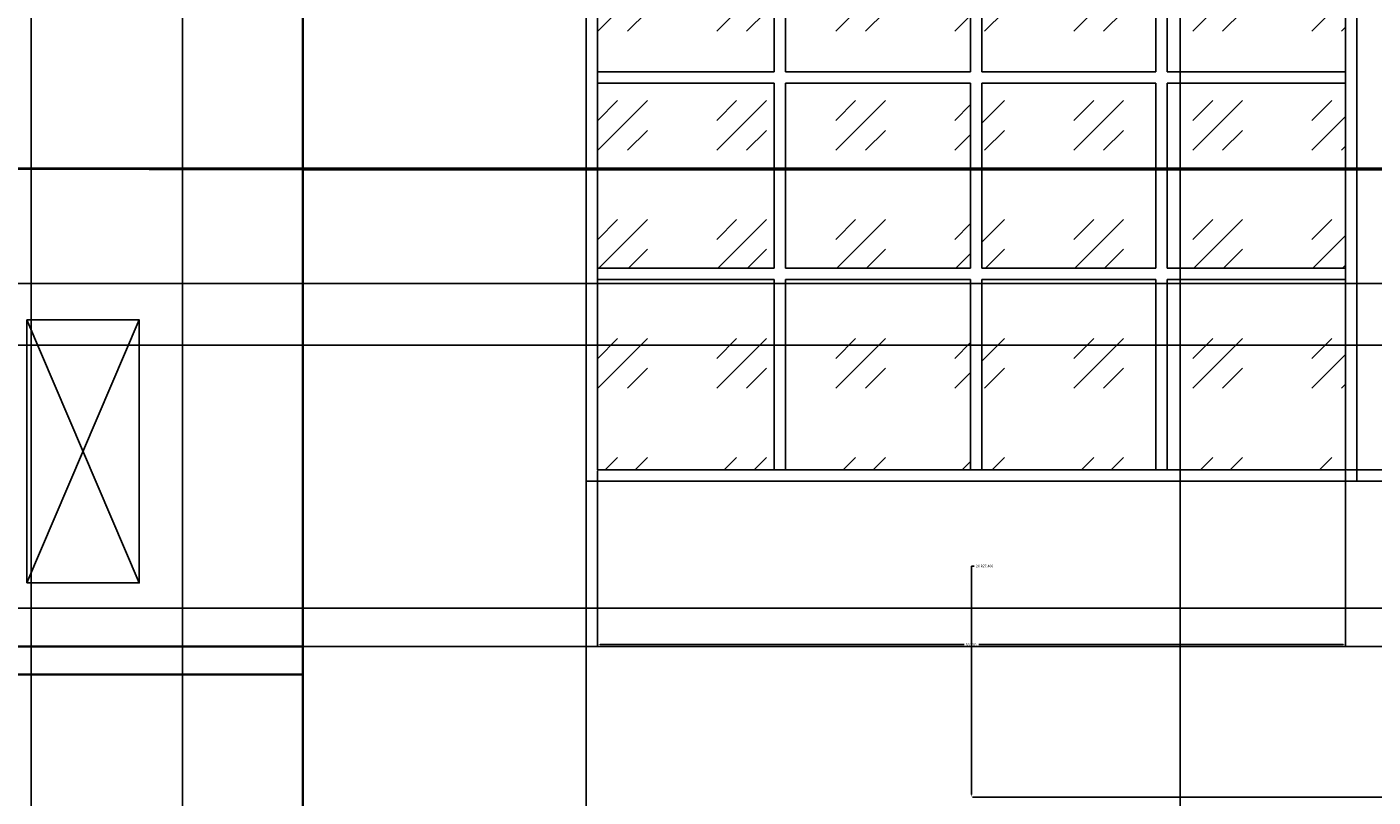
# Model space of a CAD drawing. Units: inches. Extents: x 93 to 565, y 123 to 656.
# Tile 14 of 18: x 418 to 513, y 463 to 518. Entities that reach past the tile are written whole.
import ezdxf

# ---------------------------------------------------------------- set-up
doc = ezdxf.new("R2010")
doc.units = ezdxf.units.IN
doc.header["$MEASUREMENT"] = 0
for name, color, linetype, lineweight in [('A-ANNO-DIMS', 2, 'Continuous', 18), ('A-ELEV', 7, 'Continuous', 35), ('A-GLAZ', 4, 'Continuous', 25)]:
    doc.layers.add(name, color=color, linetype=linetype, lineweight=lineweight)
doc.styles.get("Standard").update_dxf_attribs({"font": 'arial.ttf'})
doc.dimstyles.get("Standard").update_dxf_attribs({"dimtxt": 0.18, "dimasz": 0.18, "dimexe": 0.18, "dimexo": 0.0625, "dimgap": 0.09, "dimtad": 0, "dimtih": 1, "dimtoh": 1, "dimdec": 4, "dimzin": 0, "dimdsep": 46, "dimtxsty": 'Standard', "dimcen": 0.09, "dimadec": 0, "dimazin": 0, "dimtfac": 1, "dimtdec": 4, "dimtofl": 0, "dimtmove": 0, "dimatfit": 3, "dimfxl": 1, "dimtolj": 1, "dimtzin": 0, "dimarcsym": 0})

# ---------------------------------------------------------------- blocks, each defined once
blk = doc.blocks.new('*U9')
for p, q in [((0, 0), (38, 89)), ((38, 0), (0, 89))]:
    blk.add_line(p, q)
blk.add_lwpolyline([(0, 0), (38, 0), (38, 89), (0, 89)], close=True)
blk = doc.blocks.new('WIN-ARCHED')
for p, q in [((26.666, 83.051), (26.666, 70.384)), ((27.466, 83.039), (27.466, 70.358)), ((3.385, 69.387), (14.576, 63.554)), ((3.006, 68.683), (14.186, 62.855)), ((50.181, 68.96), (38.77, 63.306)), ((50.548, 68.249), (39.145, 62.599)), ((0, 56.384), (12.6, 56.384)), ((0, 56.384), (0.2, 56.384)), ((0, 56.384), (0, 32.384)), ((13.4, 56.384), (39.8, 56.384)), ((40.6, 56.384), (53.333, 56.384)), ((0, 55.584), (12.6, 55.584)), ((12.6, 55.584), (12.6, 42.384)), ((13.4, 55.584), (13.4, 42.384)), ((13.4, 55.584), (26.6, 55.584)), ((26.6, 55.584), (26.6, 42.384)), ((27.4, 55.584), (27.4, 42.384)), ((27.4, 55.584), (39.8, 55.584)), ((39.8, 55.584), (39.8, 42.384)), ((40.6, 55.584), (40.6, 42.384)), ((40.6, 55.584), (53.333, 55.584)), ((0, 42.384), (12.6, 42.384)), ((13.4, 42.384), (26.6, 42.384)), ((27.4, 42.384), (39.8, 42.384)), ((40.6, 42.384), (53.333, 42.384)), ((0, 41.584), (12.6, 41.584)), ((12.6, 41.584), (12.6, 28.384)), ((13.4, 41.584), (13.4, 28.384)), ((13.4, 41.584), (26.6, 41.584)), ((26.6, 41.584), (26.6, 28.384)), ((27.4, 41.584), (27.4, 28.384)), ((27.4, 41.584), (39.8, 41.584)), ((39.8, 41.584), (39.8, 28.384)), ((40.6, 41.584), (40.6, 28.384)), ((40.6, 41.584), (53.333, 41.584)), ((0, 28.384), (12.6, 28.384)), ((13.4, 28.384), (26.6, 28.384)), ((27.4, 28.384), (39.8, 28.384)), ((40.6, 28.384), (53.333, 28.384)), ((0, 27.584), (12.6, 27.584)), ((12.6, 27.584), (12.6, 14.384)), ((13.4, 27.584), (13.4, 14.384)), ((13.4, 27.584), (26.6, 27.584)), ((26.6, 27.584), (26.6, 14.384)), ((27.4, 27.584), (27.4, 14.384)), ((27.4, 27.584), (39.8, 27.584)), ((39.8, 27.584), (39.8, 14.384)), ((40.6, 27.584), (40.6, 14.384)), ((40.6, 27.584), (53.333, 27.584)), ((0, 14.384), (12.6, 14.384)), ((0, 13.584), (12.6, 13.584)), ((12.6, 13.584), (12.6, 0)), ((13.4, 14.384), (26.6, 14.384)), ((13.4, 13.584), (13.4, 0)), ((13.4, 13.584), (26.6, 13.584)), ((26.6, 13.584), (26.6, 0)), ((27.4, 14.384), (39.8, 14.384)), ((27.4, 13.584), (27.4, 0)), ((27.4, 13.584), (39.8, 13.584)), ((39.8, 13.584), (39.8, 0)), ((40.6, 14.384), (53.333, 14.384)), ((40.6, 13.584), (40.6, 0)), ((40.6, 13.584), (53.333, 13.584))]:
    blk.add_line(p, q)
blk.add_lwpolyline([(53.333, 56.384), (53.333, 0), (0, 0), (0, 56.384)])
for centre, radius, start, end in [((26.666, 56.384), 26.666, 90, 150.81666), ((26.666, 56.384), 26.666, 28.13721, 88.28084), ((26.6, 56.384), 14, 89.72913, 149.19423), ((26.6, 56.384), 14, 29.63071, 86.45282), ((26.6, 56.384), 13.2, 0, 180), ((26.666, 56.384), 26.666, 152.53579, 180), ((26.666, 56.384), 26.666, 0, 26.41802), ((26.6, 56.384), 14, 152.47006, 180), ((26.6, 56.384), 14, 0, 26.35489)]:
    blk.add_arc(centre, radius, start, end)
blk = doc.blocks.new('*D20')
at = {"layer": 'A-ANNO-DIMS', "color": 0, "lineweight": -2, "transparency": 16777216}
for p, q in [((511.588, 569.373), (524.163, 569.373)), ((523.983, 569.193), (523.983, 528.031)), ((523.983, 486.502), (523.983, 527.664)), ((511.588, 486.322), (524.163, 486.322))]:
    blk.add_line(p, q, dxfattribs=at)
at = {"layer": 'A-ANNO-DIMS', "color": 0, "transparency": 16777216}
for points in [[(523.953, 569.193), (524.013, 569.193), (523.983, 569.373)], [(523.953, 486.502), (524.013, 486.502), (523.983, 486.322)]]:
    blk.add_solid(points, dxfattribs=at)
at = {"layer": 'Defpoints', "color": 0, "transparency": 16777216}
for p in [(511.526, 569.373), (523.983, 569.373), (511.526, 486.322)]:
    blk.add_point(p, dxfattribs=at)
at = {"layer": 'A-ANNO-DIMS', "color": 0, "transparency": 16777216, "insert": (523.983, 527.847), "char_height": 0.18, "attachment_point": 5}
blk.add_mtext('\\A1;ARCHED WINDOW 83 TYP.', dxfattribs=at)
blk = doc.blocks.new('*D21')
at = {"layer": 'A-ANNO-DIMS', "color": 0, "lineweight": -2, "transparency": 16777216}
for p, q in [((458.193, 486.26), (458.193, 473.685)), ((511.526, 486.26), (511.526, 473.685)), ((458.373, 473.865), (484.331, 473.865)), ((511.346, 473.865), (485.388, 473.865))]:
    blk.add_line(p, q, dxfattribs=at)
at = {"layer": 'A-ANNO-DIMS', "color": 0, "transparency": 16777216}
for points in [[(458.373, 473.895), (458.373, 473.835), (458.193, 473.865)], [(511.346, 473.895), (511.346, 473.835), (511.526, 473.865)]]:
    blk.add_solid(points, dxfattribs=at)
at = {"layer": 'Defpoints', "color": 0, "transparency": 16777216}
for p in [(458.193, 486.322), (511.526, 486.322), (511.526, 473.865)]:
    blk.add_point(p, dxfattribs=at)
at = {"layer": 'A-ANNO-DIMS', "color": 0, "transparency": 16777216, "insert": (484.859, 473.865), "char_height": 0.18, "attachment_point": 5}
blk.add_mtext('\\A1;53 TYP.', dxfattribs=at)
blk = doc.blocks.new('*D29')
at = {"layer": 'A-ANNO-DIMS', "color": 0, "lineweight": -2, "transparency": 16777216}
for p, q in [((437.189, 594.342), (437.189, 134.002)), ((295.687, 183.67), (295.687, 134.002)), ((295.867, 134.182), (366.052, 134.182)), ((437.009, 134.182), (366.824, 134.182))]:
    blk.add_line(p, q, dxfattribs=at)
at = {"layer": 'A-ANNO-DIMS', "color": 0, "transparency": 16777216}
for points in [[(295.867, 134.212), (295.867, 134.152), (295.687, 134.182)], [(437.009, 134.212), (437.009, 134.152), (437.189, 134.182)]]:
    blk.add_solid(points, dxfattribs=at)
at = {"layer": 'Defpoints', "color": 0, "transparency": 16777216}
for p in [(437.189, 594.405), (295.687, 183.732), (437.189, 134.182)]:
    blk.add_point(p, dxfattribs=at)
at = {"layer": 'A-ANNO-DIMS', "color": 0, "transparency": 16777216, "insert": (366.438, 134.182), "char_height": 0.18, "attachment_point": 5}
blk.add_mtext('\\A1;141.5', dxfattribs=at)
blk = doc.blocks.new('*D30')
at = {"layer": 'A-ANNO-DIMS', "color": 0, "lineweight": -2, "transparency": 16777216}
for p, q in [((437.189, 594.342), (437.189, 134.002)), ((539.079, 159.67), (539.079, 134.002)), ((437.369, 134.182), (487.749, 134.182)), ((538.899, 134.182), (488.519, 134.182))]:
    blk.add_line(p, q, dxfattribs=at)
at = {"layer": 'A-ANNO-DIMS', "color": 0, "transparency": 16777216}
for points in [[(437.369, 134.212), (437.369, 134.152), (437.189, 134.182)], [(538.899, 134.212), (538.899, 134.152), (539.079, 134.182)]]:
    blk.add_solid(points, dxfattribs=at)
at = {"layer": 'Defpoints', "color": 0, "transparency": 16777216}
for p in [(437.189, 594.405), (539.079, 159.732), (539.079, 134.182)]:
    blk.add_point(p, dxfattribs=at)
at = {"layer": 'A-ANNO-DIMS', "color": 0, "transparency": 16777216, "insert": (488.134, 134.182), "char_height": 0.18, "attachment_point": 5}
blk.add_mtext('\\A1;101.9', dxfattribs=at)
blk = doc.blocks.new('*D31')
at = {"layer": 'A-ANNO-DIMS', "color": 0, "lineweight": -2, "transparency": 16777216}
for p, q in [((417.872, 630.405), (564.809, 630.405)), ((564.629, 630.225), (564.629, 395.25)), ((564.629, 159.912), (564.629, 394.887)), ((119.142, 159.732), (564.809, 159.732))]:
    blk.add_line(p, q, dxfattribs=at)
at = {"layer": 'A-ANNO-DIMS', "color": 0, "transparency": 16777216}
for points in [[(564.599, 630.225), (564.659, 630.225), (564.629, 630.405)], [(564.599, 159.912), (564.659, 159.912), (564.629, 159.732)]]:
    blk.add_solid(points, dxfattribs=at)
at = {"layer": 'Defpoints', "color": 0, "transparency": 16777216}
for p in [(417.81, 630.405), (564.629, 630.405), (119.079, 159.732)]:
    blk.add_point(p, dxfattribs=at)
at = {"layer": 'A-ANNO-DIMS', "color": 0, "transparency": 16777216, "insert": (564.629, 395.069), "char_height": 0.18, "attachment_point": 5}
blk.add_mtext('\\A1;470.7', dxfattribs=at)
blk = doc.blocks.new('*D69')
at = {"layer": 'A-ANNO-DIMS', "color": 0, "lineweight": -2, "transparency": 16777216}
for p, q in [((355.46, 420.63), (355.46, 656.135)), ((355.64, 655.955), (391.645, 655.955)), ((428.436, 655.955), (392.431, 655.955)), ((428.616, 420.63), (428.616, 656.135))]:
    blk.add_line(p, q, dxfattribs=at)
at = {"layer": 'A-ANNO-DIMS', "color": 0, "transparency": 16777216}
for points in [[(355.64, 655.985), (355.64, 655.925), (355.46, 655.955)], [(428.436, 655.985), (428.436, 655.925), (428.616, 655.955)]]:
    blk.add_solid(points, dxfattribs=at)
at = {"layer": 'Defpoints', "color": 0, "transparency": 16777216}
for p in [(428.616, 655.955), (355.46, 420.567), (428.616, 420.567)]:
    blk.add_point(p, dxfattribs=at)
at = {"layer": 'A-ANNO-DIMS', "color": 0, "transparency": 16777216, "insert": (392.038, 655.955), "char_height": 0.18, "attachment_point": 5}
blk.add_mtext('\\A1;73.16', dxfattribs=at)
blk = doc.blocks.new('*D73')
at = {"layer": 'A-ANNO-DIMS', "color": 0, "lineweight": -2, "transparency": 16777216}
for p, q in [((437.251, 473.732), (564.809, 473.732)), ((564.629, 473.552), (564.629, 460.914)), ((564.629, 447.912), (564.629, 460.55)), ((437.251, 447.732), (564.809, 447.732))]:
    blk.add_line(p, q, dxfattribs=at)
at = {"layer": 'A-ANNO-DIMS', "color": 0, "transparency": 16777216}
for points in [[(564.599, 473.552), (564.659, 473.552), (564.629, 473.732)], [(564.599, 447.912), (564.659, 447.912), (564.629, 447.732)]]:
    blk.add_solid(points, dxfattribs=at)
at = {"layer": 'Defpoints', "color": 0, "transparency": 16777216}
for p in [(437.189, 473.732), (564.629, 473.732), (437.189, 447.732)]:
    blk.add_point(p, dxfattribs=at)
at = {"layer": 'A-ANNO-DIMS', "color": 0, "transparency": 16777216, "insert": (564.629, 460.732), "char_height": 0.18, "attachment_point": 5}
blk.add_mtext('\\A1;26', dxfattribs=at)
blk = doc.blocks.new('*D74')
at = {"layer": 'A-ANNO-DIMS', "color": 0, "lineweight": -2, "transparency": 16777216}
for p, q in [((437.251, 507.732), (564.809, 507.732)), ((564.629, 507.552), (564.629, 490.914)), ((564.629, 473.912), (564.629, 490.55)), ((437.251, 473.732), (564.809, 473.732))]:
    blk.add_line(p, q, dxfattribs=at)
at = {"layer": 'A-ANNO-DIMS', "color": 0, "transparency": 16777216}
for points in [[(564.599, 507.552), (564.659, 507.552), (564.629, 507.732)], [(564.599, 473.912), (564.659, 473.912), (564.629, 473.732)]]:
    blk.add_solid(points, dxfattribs=at)
at = {"layer": 'Defpoints', "color": 0, "transparency": 16777216}
for p in [(437.189, 507.732), (564.629, 507.732), (437.189, 473.732)]:
    blk.add_point(p, dxfattribs=at)
at = {"layer": 'A-ANNO-DIMS', "color": 0, "transparency": 16777216, "insert": (564.629, 490.732), "char_height": 0.18, "attachment_point": 5}
blk.add_mtext('\\A1;34', dxfattribs=at)
blk = doc.blocks.new('*D76')
at = {"layer": 'A-ANNO-DIMS', "color": 0, "lineweight": -2, "transparency": 16777216}
for p, q in [((399.695, 507.892), (399.695, 656.135)), ((399.875, 655.955), (417.978, 655.955)), ((437.009, 655.955), (418.905, 655.955)), ((437.189, 507.795), (437.189, 656.135))]:
    blk.add_line(p, q, dxfattribs=at)
at = {"layer": 'A-ANNO-DIMS', "color": 0, "transparency": 16777216}
for points in [[(399.875, 655.985), (399.875, 655.925), (399.695, 655.955)], [(437.009, 655.985), (437.009, 655.925), (437.189, 655.955)]]:
    blk.add_solid(points, dxfattribs=at)
at = {"layer": 'Defpoints', "color": 0, "transparency": 16777216}
for p in [(437.189, 655.955), (399.695, 507.83), (437.189, 507.732)]:
    blk.add_point(p, dxfattribs=at)
at = {"layer": 'A-ANNO-DIMS', "color": 0, "transparency": 16777216, "insert": (418.442, 655.955), "char_height": 0.18, "attachment_point": 5}
blk.add_mtext('\\A1;37.494', dxfattribs=at)
blk = doc.blocks.new('*D77')
at = {"layer": 'A-ANNO-DIMS', "color": 0, "lineweight": -2, "transparency": 16777216}
for p, q in [((399.757, 507.83), (564.809, 507.83)), ((564.629, 507.65), (564.629, 503.901)), ((564.629, 499.789), (564.629, 503.538)), ((375.075, 499.609), (564.809, 499.609))]:
    blk.add_line(p, q, dxfattribs=at)
at = {"layer": 'A-ANNO-DIMS', "color": 0, "transparency": 16777216}
for points in [[(564.599, 507.65), (564.659, 507.65), (564.629, 507.83)], [(564.599, 499.789), (564.659, 499.789), (564.629, 499.609)]]:
    blk.add_solid(points, dxfattribs=at)
at = {"layer": 'Defpoints', "color": 0, "transparency": 16777216}
for p in [(399.695, 507.83), (564.629, 507.83), (375.012, 499.609)]:
    blk.add_point(p, dxfattribs=at)
at = {"layer": 'A-ANNO-DIMS', "color": 0, "transparency": 16777216, "insert": (564.629, 503.719), "char_height": 0.18, "attachment_point": 5}
blk.add_mtext('\\A1;8.221', dxfattribs=at)
blk = doc.blocks.new('*D79')
at = {"layer": 'A-ANNO-DIMS', "color": 0, "lineweight": -2, "transparency": 16777216}
for p, q in [((391.284, 495.217), (564.809, 495.217)), ((564.629, 495.037), (564.629, 486.022)), ((564.629, 476.644), (564.629, 485.658)), ((391.284, 476.464), (564.809, 476.464))]:
    blk.add_line(p, q, dxfattribs=at)
at = {"layer": 'A-ANNO-DIMS', "color": 0, "transparency": 16777216}
for points in [[(564.599, 495.037), (564.659, 495.037), (564.629, 495.217)], [(564.599, 476.644), (564.659, 476.644), (564.629, 476.464)]]:
    blk.add_solid(points, dxfattribs=at)
at = {"layer": 'Defpoints', "color": 0, "transparency": 16777216}
for p in [(391.222, 495.217), (564.629, 495.217), (391.222, 476.464)]:
    blk.add_point(p, dxfattribs=at)
at = {"layer": 'A-ANNO-DIMS', "color": 0, "transparency": 16777216, "insert": (564.629, 485.84), "char_height": 0.18, "attachment_point": 5}
blk.add_mtext('\\A1;18.753', dxfattribs=at)
blk = doc.blocks.new('*D82')
at = {"layer": 'A-ANNO-DIMS', "color": 0, "lineweight": -2, "transparency": 16777216}
for p, q in [((437.189, 447.795), (437.189, 656.135)), ((437.369, 655.955), (446.825, 655.955)), ((457.213, 655.955), (447.757, 655.955)), ((457.393, 378.4), (457.393, 656.135))]:
    blk.add_line(p, q, dxfattribs=at)
at = {"layer": 'A-ANNO-DIMS', "color": 0, "transparency": 16777216}
for points in [[(437.369, 655.985), (437.369, 655.925), (437.189, 655.955)], [(457.213, 655.985), (457.213, 655.925), (457.393, 655.955)]]:
    blk.add_solid(points, dxfattribs=at)
at = {"layer": 'Defpoints', "color": 0, "transparency": 16777216}
for p in [(457.393, 655.955), (437.189, 447.732), (457.393, 378.337)]:
    blk.add_point(p, dxfattribs=at)
at = {"layer": 'A-ANNO-DIMS', "color": 0, "transparency": 16777216, "insert": (447.291, 655.955), "char_height": 0.18, "attachment_point": 5}
blk.add_mtext('\\A1;20.205', dxfattribs=at)
blk = doc.blocks.new('*D85')
at = {"layer": 'A-ANNO-DIMS', "color": 0, "lineweight": -2, "transparency": 16777216}
for p, q in [((457.456, 485.522), (564.809, 485.522)), ((564.629, 485.342), (564.629, 474.437)), ((564.629, 463.168), (564.629, 474.073)), ((484.922, 462.988), (564.809, 462.988))]:
    blk.add_line(p, q, dxfattribs=at)
at = {"layer": 'A-ANNO-DIMS', "color": 0, "transparency": 16777216}
for points in [[(564.599, 485.342), (564.659, 485.342), (564.629, 485.522)], [(564.599, 463.168), (564.659, 463.168), (564.629, 462.988)]]:
    blk.add_solid(points, dxfattribs=at)
at = {"layer": 'Defpoints', "color": 0, "transparency": 16777216}
for p in [(457.393, 485.522), (564.629, 485.522), (484.859, 462.988)]:
    blk.add_point(p, dxfattribs=at)
at = {"layer": 'A-ANNO-DIMS', "color": 0, "transparency": 16777216, "insert": (564.629, 474.255), "char_height": 0.18, "attachment_point": 5}
blk.add_mtext('\\A1;22.535', dxfattribs=at)
blk = doc.blocks.new('*D90')
at = {"layer": 'A-ANNO-DIMS', "color": 0, "lineweight": -2, "transparency": 16777216}
for p, q in [((417.81, 594.342), (417.81, 134.002)), ((437.189, 594.342), (437.189, 134.002)), ((417.99, 134.182), (427.114, 134.182)), ((437.009, 134.182), (427.885, 134.182))]:
    blk.add_line(p, q, dxfattribs=at)
at = {"layer": 'A-ANNO-DIMS', "color": 0, "transparency": 16777216}
for points in [[(417.99, 134.212), (417.99, 134.152), (417.81, 134.182)], [(437.009, 134.212), (437.009, 134.152), (437.189, 134.182)]]:
    blk.add_solid(points, dxfattribs=at)
at = {"layer": 'Defpoints', "color": 0, "transparency": 16777216}
for p in [(417.81, 594.405), (437.189, 594.405), (437.189, 134.182)]:
    blk.add_point(p, dxfattribs=at)
at = {"layer": 'A-ANNO-DIMS', "color": 0, "transparency": 16777216, "insert": (427.499, 134.182), "char_height": 0.18, "attachment_point": 5}
blk.add_mtext('\\A1;19.38', dxfattribs=at)
blk = doc.blocks.new('*D91')
at = {"layer": 'A-ANNO-DIMS', "color": 0, "lineweight": -2, "transparency": 16777216}
for p, q in [((499.729, 599.755), (499.729, 134.002)), ((437.189, 594.342), (437.189, 134.002)), ((437.369, 134.182), (468.065, 134.182)), ((499.549, 134.182), (468.853, 134.182))]:
    blk.add_line(p, q, dxfattribs=at)
at = {"layer": 'A-ANNO-DIMS', "color": 0, "transparency": 16777216}
for points in [[(437.369, 134.212), (437.369, 134.152), (437.189, 134.182)], [(499.549, 134.212), (499.549, 134.152), (499.729, 134.182)]]:
    blk.add_solid(points, dxfattribs=at)
at = {"layer": 'Defpoints', "color": 0, "transparency": 16777216}
for p in [(499.729, 599.817), (437.189, 594.405), (499.729, 134.182)]:
    blk.add_point(p, dxfattribs=at)
at = {"layer": 'A-ANNO-DIMS', "color": 0, "transparency": 16777216, "insert": (468.459, 134.182), "char_height": 0.18, "attachment_point": 5}
blk.add_mtext('\\A1;62.54', dxfattribs=at)
blk = doc.blocks.new('*D92')
at = {"layer": 'A-ANNO-DIMS', "color": 0, "lineweight": -2, "transparency": 16777216}
for p, q in [((523.142, 603.135), (523.142, 134.002)), ((499.729, 599.755), (499.729, 134.002)), ((499.909, 134.182), (510.971, 134.182)), ((522.962, 134.182), (511.9, 134.182))]:
    blk.add_line(p, q, dxfattribs=at)
at = {"layer": 'A-ANNO-DIMS', "color": 0, "transparency": 16777216}
for points in [[(499.909, 134.212), (499.909, 134.152), (499.729, 134.182)], [(522.962, 134.212), (522.962, 134.152), (523.142, 134.182)]]:
    blk.add_solid(points, dxfattribs=at)
at = {"layer": 'Defpoints', "color": 0, "transparency": 16777216}
for p in [(523.142, 603.198), (499.729, 599.817), (523.142, 134.182)]:
    blk.add_point(p, dxfattribs=at)
at = {"layer": 'A-ANNO-DIMS', "color": 0, "transparency": 16777216, "insert": (511.435, 134.182), "char_height": 0.18, "attachment_point": 5}
blk.add_mtext('\\A1;23.412', dxfattribs=at)
blk = doc.blocks.new('*D101')
at = {"layer": 'A-ANNO-DIMS', "color": 0, "lineweight": -2, "transparency": 16777216}
for p, q in [((485.04, 479.467), (484.86, 479.467)), ((484.86, 479.467), (484.86, 463.168)), ((484.769, 435.521), (484.949, 435.521)), ((484.859, 435.431), (484.859, 435.611))]:
    blk.add_line(p, q, dxfattribs=at)
at = {"layer": 'A-ANNO-DIMS', "color": 0, "transparency": 16777216}
blk.add_solid([(484.83, 463.168), (484.89, 463.168), (484.86, 462.988)], dxfattribs=at)
at = {"layer": 'Defpoints', "color": 0, "transparency": 16777216}
for p in [(484.86, 462.988), (484.859, 435.521)]:
    blk.add_point(p, dxfattribs=at)
at = {"layer": 'A-ANNO-DIMS', "color": 0, "transparency": 16777216, "insert": (485.785, 479.467), "char_height": 0.18, "attachment_point": 5}
blk.add_mtext('\\A1;2X R27.466', dxfattribs=at)
blk = doc.blocks.new('*D108')
at = {"layer": 'A-ANNO-DIMS', "color": 0, "lineweight": -2, "transparency": 16777216}
for p, q in [((437.189, 594.342), (437.189, 134.002)), ((295.687, 183.67), (295.687, 134.002)), ((295.867, 134.182), (365.93, 134.182)), ((437.009, 134.182), (366.946, 134.182))]:
    blk.add_line(p, q, dxfattribs=at)
at = {"layer": 'A-ANNO-DIMS', "color": 0, "transparency": 16777216}
for points in [[(295.867, 134.212), (295.867, 134.152), (295.687, 134.182)], [(437.009, 134.212), (437.009, 134.152), (437.189, 134.182)]]:
    blk.add_solid(points, dxfattribs=at)
at = {"layer": 'Defpoints', "color": 0, "transparency": 16777216}
for p in [(437.189, 594.405), (295.687, 183.732), (437.189, 134.182)]:
    blk.add_point(p, dxfattribs=at)
at = {"layer": 'A-ANNO-DIMS', "color": 0, "transparency": 16777216, "insert": (366.438, 134.182), "char_height": 0.18, "attachment_point": 5}
blk.add_mtext('\\A1;141.501', dxfattribs=at)
blk = doc.blocks.new('*D109')
at = {"layer": 'A-ANNO-DIMS', "color": 0, "lineweight": -2, "transparency": 16777216}
for p, q in [((437.189, 594.342), (437.189, 134.002)), ((539.079, 159.67), (539.079, 134.002)), ((437.369, 134.182), (487.626, 134.182)), ((538.899, 134.182), (488.642, 134.182))]:
    blk.add_line(p, q, dxfattribs=at)
at = {"layer": 'A-ANNO-DIMS', "color": 0, "transparency": 16777216}
for points in [[(437.369, 134.212), (437.369, 134.152), (437.189, 134.182)], [(538.899, 134.212), (538.899, 134.152), (539.079, 134.182)]]:
    blk.add_solid(points, dxfattribs=at)
at = {"layer": 'Defpoints', "color": 0, "transparency": 16777216}
for p in [(437.189, 594.405), (539.079, 159.732), (539.079, 134.182)]:
    blk.add_point(p, dxfattribs=at)
at = {"layer": 'A-ANNO-DIMS', "color": 0, "transparency": 16777216, "insert": (488.134, 134.182), "char_height": 0.18, "attachment_point": 5}
blk.add_mtext('\\A1;101.891', dxfattribs=at)
blk = doc.blocks.new('*D110')
at = {"layer": 'A-ANNO-DIMS', "color": 0, "lineweight": -2, "transparency": 16777216}
for p, q in [((417.872, 630.405), (564.809, 630.405)), ((564.629, 630.225), (564.629, 395.25)), ((564.629, 159.912), (564.629, 394.887)), ((119.142, 159.732), (564.809, 159.732))]:
    blk.add_line(p, q, dxfattribs=at)
at = {"layer": 'A-ANNO-DIMS', "color": 0, "transparency": 16777216}
for points in [[(564.599, 630.225), (564.659, 630.225), (564.629, 630.405)], [(564.599, 159.912), (564.659, 159.912), (564.629, 159.732)]]:
    blk.add_solid(points, dxfattribs=at)
at = {"layer": 'Defpoints', "color": 0, "transparency": 16777216}
for p in [(417.81, 630.405), (564.629, 630.405), (119.079, 159.732)]:
    blk.add_point(p, dxfattribs=at)
at = {"layer": 'A-ANNO-DIMS', "color": 0, "transparency": 16777216, "insert": (564.629, 395.069), "char_height": 0.18, "attachment_point": 5}
blk.add_mtext('\\A1;470.673', dxfattribs=at)
blk = doc.blocks.new('*D148')
at = {"layer": 'A-ANNO-DIMS', "color": 0, "lineweight": -2, "transparency": 16777216}
for p, q in [((355.46, 420.63), (355.46, 656.135)), ((355.64, 655.955), (391.575, 655.955)), ((428.436, 655.955), (392.501, 655.955)), ((428.616, 420.63), (428.616, 656.135))]:
    blk.add_line(p, q, dxfattribs=at)
at = {"layer": 'A-ANNO-DIMS', "color": 0, "transparency": 16777216}
for points in [[(355.64, 655.985), (355.64, 655.925), (355.46, 655.955)], [(428.436, 655.985), (428.436, 655.925), (428.616, 655.955)]]:
    blk.add_solid(points, dxfattribs=at)
at = {"layer": 'Defpoints', "color": 0, "transparency": 16777216}
for p in [(428.616, 655.955), (355.46, 420.567), (428.616, 420.567)]:
    blk.add_point(p, dxfattribs=at)
at = {"layer": 'A-ANNO-DIMS', "color": 0, "transparency": 16777216, "insert": (392.038, 655.955), "char_height": 0.18, "attachment_point": 5}
blk.add_mtext('\\A1;73.156', dxfattribs=at)
blk = doc.blocks.new('*D152')
at = {"layer": 'A-ANNO-DIMS', "color": 0, "lineweight": -2, "transparency": 16777216}
for p, q in [((437.251, 473.732), (564.809, 473.732)), ((564.629, 473.552), (564.629, 460.914)), ((564.629, 447.912), (564.629, 460.55)), ((437.251, 447.732), (564.809, 447.732))]:
    blk.add_line(p, q, dxfattribs=at)
at = {"layer": 'A-ANNO-DIMS', "color": 0, "transparency": 16777216}
for points in [[(564.599, 473.552), (564.659, 473.552), (564.629, 473.732)], [(564.599, 447.912), (564.659, 447.912), (564.629, 447.732)]]:
    blk.add_solid(points, dxfattribs=at)
at = {"layer": 'Defpoints', "color": 0, "transparency": 16777216}
for p in [(437.189, 473.732), (564.629, 473.732), (437.189, 447.732)]:
    blk.add_point(p, dxfattribs=at)
at = {"layer": 'A-ANNO-DIMS', "color": 0, "transparency": 16777216, "insert": (564.629, 460.732), "char_height": 0.18, "attachment_point": 5}
blk.add_mtext('\\A1;26.000', dxfattribs=at)
blk = doc.blocks.new('*D153')
at = {"layer": 'A-ANNO-DIMS', "color": 0, "lineweight": -2, "transparency": 16777216}
for p, q in [((437.251, 507.732), (564.809, 507.732)), ((564.629, 507.552), (564.629, 490.914)), ((564.629, 473.912), (564.629, 490.55)), ((437.251, 473.732), (564.809, 473.732))]:
    blk.add_line(p, q, dxfattribs=at)
at = {"layer": 'A-ANNO-DIMS', "color": 0, "transparency": 16777216}
for points in [[(564.599, 507.552), (564.659, 507.552), (564.629, 507.732)], [(564.599, 473.912), (564.659, 473.912), (564.629, 473.732)]]:
    blk.add_solid(points, dxfattribs=at)
at = {"layer": 'Defpoints', "color": 0, "transparency": 16777216}
for p in [(437.189, 507.732), (564.629, 507.732), (437.189, 473.732)]:
    blk.add_point(p, dxfattribs=at)
at = {"layer": 'A-ANNO-DIMS', "color": 0, "transparency": 16777216, "insert": (564.629, 490.732), "char_height": 0.18, "attachment_point": 5}
blk.add_mtext('\\A1;34.000', dxfattribs=at)
blk = doc.blocks.new('*D155')
at = {"layer": 'A-ANNO-DIMS', "color": 0, "lineweight": -2, "transparency": 16777216}
for p, q in [((399.695, 507.892), (399.695, 656.135)), ((399.875, 655.955), (417.978, 655.955)), ((437.009, 655.955), (418.905, 655.955)), ((437.189, 507.795), (437.189, 656.135))]:
    blk.add_line(p, q, dxfattribs=at)
at = {"layer": 'A-ANNO-DIMS', "color": 0, "transparency": 16777216}
for points in [[(399.875, 655.985), (399.875, 655.925), (399.695, 655.955)], [(437.009, 655.985), (437.009, 655.925), (437.189, 655.955)]]:
    blk.add_solid(points, dxfattribs=at)
at = {"layer": 'Defpoints', "color": 0, "transparency": 16777216}
for p in [(437.189, 655.955), (399.695, 507.83), (437.189, 507.732)]:
    blk.add_point(p, dxfattribs=at)
at = {"layer": 'A-ANNO-DIMS', "color": 0, "transparency": 16777216, "insert": (418.442, 655.955), "char_height": 0.18, "attachment_point": 5}
blk.add_mtext('\\A1;37.494', dxfattribs=at)
blk = doc.blocks.new('*D156')
at = {"layer": 'A-ANNO-DIMS', "color": 0, "lineweight": -2, "transparency": 16777216}
for p, q in [((399.757, 507.83), (564.809, 507.83)), ((564.629, 507.65), (564.629, 503.901)), ((564.629, 499.789), (564.629, 503.538)), ((375.075, 499.609), (564.809, 499.609))]:
    blk.add_line(p, q, dxfattribs=at)
at = {"layer": 'A-ANNO-DIMS', "color": 0, "transparency": 16777216}
for points in [[(564.599, 507.65), (564.659, 507.65), (564.629, 507.83)], [(564.599, 499.789), (564.659, 499.789), (564.629, 499.609)]]:
    blk.add_solid(points, dxfattribs=at)
at = {"layer": 'Defpoints', "color": 0, "transparency": 16777216}
for p in [(399.695, 507.83), (564.629, 507.83), (375.012, 499.609)]:
    blk.add_point(p, dxfattribs=at)
at = {"layer": 'A-ANNO-DIMS', "color": 0, "transparency": 16777216, "insert": (564.629, 503.719), "char_height": 0.18, "attachment_point": 5}
blk.add_mtext('\\A1;8.221', dxfattribs=at)
blk = doc.blocks.new('*D158')
at = {"layer": 'A-ANNO-DIMS', "color": 0, "lineweight": -2, "transparency": 16777216}
for p, q in [((391.284, 495.217), (564.809, 495.217)), ((564.629, 495.037), (564.629, 486.022)), ((564.629, 476.644), (564.629, 485.658)), ((391.284, 476.464), (564.809, 476.464))]:
    blk.add_line(p, q, dxfattribs=at)
at = {"layer": 'A-ANNO-DIMS', "color": 0, "transparency": 16777216}
for points in [[(564.599, 495.037), (564.659, 495.037), (564.629, 495.217)], [(564.599, 476.644), (564.659, 476.644), (564.629, 476.464)]]:
    blk.add_solid(points, dxfattribs=at)
at = {"layer": 'Defpoints', "color": 0, "transparency": 16777216}
for p in [(391.222, 495.217), (564.629, 495.217), (391.222, 476.464)]:
    blk.add_point(p, dxfattribs=at)
at = {"layer": 'A-ANNO-DIMS', "color": 0, "transparency": 16777216, "insert": (564.629, 485.84), "char_height": 0.18, "attachment_point": 5}
blk.add_mtext('\\A1;18.753', dxfattribs=at)
blk = doc.blocks.new('*D161')
at = {"layer": 'A-ANNO-DIMS', "color": 0, "lineweight": -2, "transparency": 16777216}
for p, q in [((437.189, 447.795), (437.189, 656.135)), ((437.369, 655.955), (446.825, 655.955)), ((457.213, 655.955), (447.757, 655.955)), ((457.393, 378.4), (457.393, 656.135))]:
    blk.add_line(p, q, dxfattribs=at)
at = {"layer": 'A-ANNO-DIMS', "color": 0, "transparency": 16777216}
for points in [[(437.369, 655.985), (437.369, 655.925), (437.189, 655.955)], [(457.213, 655.985), (457.213, 655.925), (457.393, 655.955)]]:
    blk.add_solid(points, dxfattribs=at)
at = {"layer": 'Defpoints', "color": 0, "transparency": 16777216}
for p in [(457.393, 655.955), (437.189, 447.732), (457.393, 378.337)]:
    blk.add_point(p, dxfattribs=at)
at = {"layer": 'A-ANNO-DIMS', "color": 0, "transparency": 16777216, "insert": (447.291, 655.955), "char_height": 0.18, "attachment_point": 5}
blk.add_mtext('\\A1;20.205', dxfattribs=at)
blk = doc.blocks.new('*D164')
at = {"layer": 'A-ANNO-DIMS', "color": 0, "lineweight": -2, "transparency": 16777216}
for p, q in [((457.456, 485.522), (564.809, 485.522)), ((564.629, 485.342), (564.629, 474.437)), ((564.629, 463.168), (564.629, 474.073)), ((484.922, 462.988), (564.809, 462.988))]:
    blk.add_line(p, q, dxfattribs=at)
at = {"layer": 'A-ANNO-DIMS', "color": 0, "transparency": 16777216}
for points in [[(564.599, 485.342), (564.659, 485.342), (564.629, 485.522)], [(564.599, 463.168), (564.659, 463.168), (564.629, 462.988)]]:
    blk.add_solid(points, dxfattribs=at)
at = {"layer": 'Defpoints', "color": 0, "transparency": 16777216}
for p in [(457.393, 485.522), (564.629, 485.522), (484.859, 462.988)]:
    blk.add_point(p, dxfattribs=at)
at = {"layer": 'A-ANNO-DIMS', "color": 0, "transparency": 16777216, "insert": (564.629, 474.255), "char_height": 0.18, "attachment_point": 5}
blk.add_mtext('\\A1;22.535', dxfattribs=at)
blk = doc.blocks.new('*D169')
at = {"layer": 'A-ANNO-DIMS', "color": 0, "lineweight": -2, "transparency": 16777216}
for p, q in [((417.81, 594.342), (417.81, 134.002)), ((437.189, 594.342), (437.189, 134.002)), ((417.99, 134.182), (427.044, 134.182)), ((437.009, 134.182), (427.954, 134.182))]:
    blk.add_line(p, q, dxfattribs=at)
at = {"layer": 'A-ANNO-DIMS', "color": 0, "transparency": 16777216}
for points in [[(417.99, 134.212), (417.99, 134.152), (417.81, 134.182)], [(437.009, 134.212), (437.009, 134.152), (437.189, 134.182)]]:
    blk.add_solid(points, dxfattribs=at)
at = {"layer": 'Defpoints', "color": 0, "transparency": 16777216}
for p in [(417.81, 594.405), (437.189, 594.405), (437.189, 134.182)]:
    blk.add_point(p, dxfattribs=at)
at = {"layer": 'A-ANNO-DIMS', "color": 0, "transparency": 16777216, "insert": (427.499, 134.182), "char_height": 0.18, "attachment_point": 5}
blk.add_mtext('\\A1;19.379', dxfattribs=at)
blk = doc.blocks.new('*D170')
at = {"layer": 'A-ANNO-DIMS', "color": 0, "lineweight": -2, "transparency": 16777216}
for p, q in [((499.729, 599.755), (499.729, 134.002)), ((437.189, 594.342), (437.189, 134.002)), ((437.369, 134.182), (468.012, 134.182)), ((499.549, 134.182), (468.906, 134.182))]:
    blk.add_line(p, q, dxfattribs=at)
at = {"layer": 'A-ANNO-DIMS', "color": 0, "transparency": 16777216}
for points in [[(437.369, 134.212), (437.369, 134.152), (437.189, 134.182)], [(499.549, 134.212), (499.549, 134.152), (499.729, 134.182)]]:
    blk.add_solid(points, dxfattribs=at)
at = {"layer": 'Defpoints', "color": 0, "transparency": 16777216}
for p in [(499.729, 599.817), (437.189, 594.405), (499.729, 134.182)]:
    blk.add_point(p, dxfattribs=at)
at = {"layer": 'A-ANNO-DIMS', "color": 0, "transparency": 16777216, "insert": (468.459, 134.182), "char_height": 0.18, "attachment_point": 5}
blk.add_mtext('\\A1;62.541', dxfattribs=at)
blk = doc.blocks.new('*D171')
at = {"layer": 'A-ANNO-DIMS', "color": 0, "lineweight": -2, "transparency": 16777216}
for p, q in [((523.142, 603.135), (523.142, 134.002)), ((499.729, 599.755), (499.729, 134.002)), ((499.909, 134.182), (510.971, 134.182)), ((522.962, 134.182), (511.9, 134.182))]:
    blk.add_line(p, q, dxfattribs=at)
at = {"layer": 'A-ANNO-DIMS', "color": 0, "transparency": 16777216}
for points in [[(499.909, 134.212), (499.909, 134.152), (499.729, 134.182)], [(522.962, 134.212), (522.962, 134.152), (523.142, 134.182)]]:
    blk.add_solid(points, dxfattribs=at)
at = {"layer": 'Defpoints', "color": 0, "transparency": 16777216}
for p in [(523.142, 603.198), (499.729, 599.817), (523.142, 134.182)]:
    blk.add_point(p, dxfattribs=at)
at = {"layer": 'A-ANNO-DIMS', "color": 0, "transparency": 16777216, "insert": (511.435, 134.182), "char_height": 0.18, "attachment_point": 5}
blk.add_mtext('\\A1;23.412', dxfattribs=at)
blk = doc.blocks.new('*D199')
at = {"layer": 'A-ANNO-DIMS', "color": 0, "lineweight": -2, "transparency": 16777216}
for p, q in [((485.04, 479.467), (484.86, 479.467)), ((484.86, 479.467), (484.86, 463.168)), ((484.769, 435.521), (484.949, 435.521)), ((484.859, 435.431), (484.859, 435.611))]:
    blk.add_line(p, q, dxfattribs=at)
at = {"layer": 'A-ANNO-DIMS', "color": 0, "transparency": 16777216}
blk.add_solid([(484.83, 463.168), (484.89, 463.168), (484.86, 462.988)], dxfattribs=at)
at = {"layer": 'Defpoints', "color": 0, "transparency": 16777216}
for p in [(484.86, 462.988), (484.859, 435.521)]:
    blk.add_point(p, dxfattribs=at)
at = {"layer": 'A-ANNO-DIMS', "color": 0, "transparency": 16777216, "insert": (485.785, 479.467), "char_height": 0.18, "attachment_point": 5}
blk.add_mtext('\\A1;2X R27.466', dxfattribs=at)

msp = doc.modelspace()

# ---------------------------------------------------------------- hatches: boundary and pattern name
at = {"layer": 'A-GLAZ'}
h = msp.add_hatch(dxfattribs=at)
h.set_pattern_fill('GOST_GLASS', color=256)
h.set_pattern_definition([(45, (0, 0), (8.48528, 0), [5, -7]), (45, (2.1213, 0), (8.48528, 0), [2, -10]), (45, (0, 2.1213), (8.48528, 0), [2, -10])])
h.paths.add_polyline_path([(472.3785, 549.1774), (461.1986, 555.0047, 0.1204122), (458.1933, 542.7064), (458.3933, 542.7064), (470.7933, 542.7064, -0.1207031)])
h.paths.add_polyline_path([(470.7933, 541.9064), (458.1933, 541.9064), (458.1933, 528.7064), (470.7933, 528.7064)])
h.paths.add_polyline_path([(470.7933, 527.9064), (458.1933, 527.9064), (458.1933, 518.7064), (458.1933, 514.7064), (470.7933, 514.7064)])
h.paths.add_polyline_path([(470.7933, 513.9064), (458.1933, 513.9064), (458.1933, 500.7064), (470.7933, 500.7064)])
h.paths.add_polyline_path([(470.7933, 499.9064), (458.1933, 499.9064), (458.1933, 486.3222), (470.7933, 486.3222)])
h.paths.add_polyline_path([(484.7933, 499.9064), (471.5933, 499.9064), (471.5933, 486.3222), (484.7933, 486.3222)])
h.paths.add_polyline_path([(484.7933, 513.9064), (471.5933, 513.9064), (471.5933, 500.7064), (484.7933, 500.7064)])
h.paths.add_polyline_path([(484.7933, 527.9064), (471.5933, 527.9064), (471.5933, 514.7064), (484.7933, 514.7064)])
h.paths.add_polyline_path([(484.7933, 541.9064), (471.5933, 541.9064), (471.5933, 528.7064), (484.7933, 528.7064)])
h.paths.add_polyline_path([(497.9933, 541.9064), (485.5933, 541.9064), (485.5933, 528.7064), (497.9933, 528.7064)])
h.paths.add_polyline_path([(497.9933, 527.9064), (485.5933, 527.9064), (485.5933, 514.7064), (497.9933, 514.7064)])
h.paths.add_polyline_path([(497.9933, 513.9064), (485.5933, 513.9064), (485.5933, 500.7064), (497.9933, 500.7064)])
h.paths.add_polyline_path([(497.9933, 499.9064), (485.5933, 499.9064), (485.5933, 486.3222), (497.9933, 486.3222)])
h.paths.add_polyline_path([(511.5257, 499.9064), (498.7933, 499.9064), (498.7933, 486.3222), (511.5257, 486.3222)])
h.paths.add_polyline_path([(511.5257, 513.9064), (498.7933, 513.9064), (498.7933, 500.7064), (511.5257, 500.7064)])
h.paths.add_polyline_path([(511.5257, 527.9064), (498.7933, 527.9064), (498.7933, 514.7064), (511.5257, 514.7064)])
h.paths.add_polyline_path([(511.5257, 541.9064), (498.7933, 541.9064), (498.7933, 528.7064), (511.5257, 528.7064)])
h.paths.add_polyline_path([(471.5933, 542.7064), (497.9933, 542.7064, 1)])
h.paths.add_polyline_path([(508.741, 554.5706), (497.3382, 548.9214, -0.1155045), (498.7933, 542.7064), (511.5257, 542.7064, 0.1157836)])
h.paths.add_polyline_path([(485.6595, 569.3606), (485.6595, 556.6796, -0.2531415), (496.9625, 549.6281), (508.3743, 555.2818, 0.268621)])
h.paths.add_polyline_path([(484.8595, 569.3726, 0.271772), (461.5782, 555.709), (472.7686, 549.8762, -0.2654493), (484.8595, 556.7062)])

# ---------------------------------------------------------------- linework, layer by layer
at = {"layer": 'A-ELEV'}
for p, q in [((437.1885, 594.4048), (437.1885, 507.7323)), ((399.6946, 507.8299), (437.1885, 507.7323)), ((437.1885, 507.7323), (437.1885, 447.7323)), ((210.5443, 473.7323), (437.1885, 473.7323)), ((210.5443, 471.7323), (437.1885, 471.7323))]:
    msp.add_line(p, q, dxfattribs=at)
at = {"layer": 'A-GLAZ'}
msp.add_lwpolyline([(512.3257, 542.7064), (512.3257, 485.5222), (457.3933, 485.5222), (457.3933, 542.7064)], dxfattribs=at)

# ---------------------------------------------------------------- block references
msp.add_blockref('WIN-ARCHED', (458.193, 486.322), dxfattribs=at)
at = {"layer": 'A-GLAZ', "xscale": 0.2107133031769033, "yscale": 0.2107133031769033, "zscale": 0.2107133031769033}
msp.add_blockref('*U9', (417.5132, 478.2628), dxfattribs=at)

# ---------------------------------------------------------------- dimensions: what is measured, and where the dimension line sits
at = {"layer": 'A-ANNO-DIMS'}
for base, p1, p2, override, picture, middle in [((428.6158, 655.9548), (355.4603, 420.5674), (428.6158, 420.5674), {"dimdec": 2, "dimlfac": 1, "dimrnd": 0, "dimzin": 0, "dimdsep": 46, "dimlunit": 2}, '*D69', (392.038, 655.9548)), ((428.615792, 655.954775), (355.460288, 420.567351), (428.615792, 420.567351), {"dimdec": 3, "dimlfac": 1, "dimrnd": 0, "dimzin": 0, "dimdsep": 46, "dimlunit": 2}, '*D148', (392.03804, 655.954775)), ((437.1885, 655.9548), (399.6946, 507.8299), (437.1885, 507.7323), {"dimdec": 3, "dimlfac": 1, "dimrnd": 0, "dimzin": 0, "dimdsep": 46, "dimlunit": 2}, '*D76', (418.4415, 655.9548)), ((437.1885, 655.9548), (399.6946, 507.8299), (437.1885, 507.7323), {"dimdec": 3, "dimlfac": 1, "dimrnd": 0, "dimzin": 0, "dimdsep": 46, "dimlunit": 2}, '*D155', (418.4415, 655.9548)), ((457.3933, 655.9548), (437.1885, 447.7323), (457.3933, 378.3372), {"dimdec": 3, "dimlfac": 1, "dimrnd": 0, "dimzin": 0, "dimdsep": 46, "dimlunit": 2}, '*D82', (447.2909, 655.9548)), ((457.3933, 655.9548), (437.1885, 447.7323), (457.3933, 378.3372), {"dimdec": 3, "dimlfac": 1, "dimrnd": 0, "dimzin": 0, "dimdsep": 46, "dimlunit": 2}, '*D161', (447.2909, 655.9548)), ((523.1415, 134.1823), (499.7291, 599.8171), (523.1415, 603.1979), {"dimdec": 3, "dimlfac": 1, "dimrnd": 0, "dimzin": 0, "dimdsep": 46, "dimlunit": 2}, '*D92', (511.4353, 134.1823)), ((523.1415, 134.1823), (499.7291, 599.8171), (523.1415, 603.1979), {"dimdec": 3, "dimlfac": 1, "dimrnd": 0, "dimzin": 0, "dimdsep": 46, "dimlunit": 2}, '*D171', (511.4353, 134.1823)), ((499.7291, 134.1823), (437.1885, 594.4048), (499.7291, 599.8171), {"dimdec": 2, "dimlfac": 1, "dimrnd": 0, "dimzin": 0, "dimdsep": 46, "dimlunit": 2}, '*D91', (468.4588, 134.1823)), ((499.7291, 134.1823), (437.1885, 594.4048), (499.7291, 599.8171), {"dimdec": 3, "dimlfac": 1, "dimrnd": 0, "dimzin": 0, "dimdsep": 46, "dimlunit": 2}, '*D170', (468.4588, 134.1823)), ((437.1885, 134.1823), (295.6874, 183.7323), (437.1885, 594.4048), {"dimdec": 1, "dimlfac": 1, "dimrnd": 0, "dimzin": 0, "dimdsep": 46, "dimlunit": 2}, '*D29', (366.438, 134.1823)), ((437.1885, 134.1823), (295.6874, 183.7323), (437.1885, 594.4048), {"dimdec": 3, "dimlfac": 1, "dimrnd": 0, "dimzin": 0, "dimdsep": 46, "dimlunit": 2}, '*D108', (366.438, 134.1823)), ((437.1885, 134.1823), (417.8097, 594.4048), (437.1885, 594.4048), {"dimdec": 2, "dimlfac": 1, "dimrnd": 0, "dimzin": 0, "dimdsep": 46, "dimlunit": 2}, '*D90', (427.4991, 134.1823)), ((437.1885, 134.1823), (417.8097, 594.4048), (437.1885, 594.4048), {"dimdec": 3, "dimlfac": 1, "dimrnd": 0, "dimzin": 0, "dimdsep": 46, "dimlunit": 2}, '*D169', (427.4991, 134.1823)), ((539.0794, 134.1823), (437.1885, 594.4048), (539.0794, 159.7323), {"dimdec": 1, "dimlfac": 1, "dimrnd": 0, "dimzin": 0, "dimdsep": 46, "dimlunit": 2}, '*D30', (488.1339, 134.1823)), ((539.0794, 134.1823), (437.1885, 594.4048), (539.0794, 159.7323), {"dimdec": 3, "dimlfac": 1, "dimrnd": 0, "dimzin": 0, "dimdsep": 46, "dimlunit": 2}, '*D109', (488.1339, 134.1823))]:
    dim = msp.add_linear_dim(base=base, p1=p1, p2=p2, dimstyle='Standard', override=override, dxfattribs=at)
    dim.commit()
    dim.dimension.update_dxf_attribs({"geometry": picture, "text_midpoint": middle})
for base, p1, p2, override, picture, middle in [((564.6294, 630.4048), (119.0794, 159.7323), (417.8097, 630.4048), {"dimdec": 1, "dimlfac": 1, "dimrnd": 0, "dimzin": 0, "dimdsep": 46, "dimlunit": 2}, '*D31', (564.6294, 395.0685)), ((564.62936, 630.40478), (119.07936, 159.73225), (417.80971, 630.40477), {"dimdec": 3, "dimlfac": 1, "dimrnd": 0, "dimzin": 0, "dimdsep": 46, "dimlunit": 2}, '*D110', (564.62936, 395.06851)), ((564.6294, 507.8299), (375.0121, 499.609), (399.6946, 507.8299), {"dimdec": 3, "dimlfac": 1, "dimrnd": 0, "dimzin": 0, "dimdsep": 46, "dimlunit": 2}, '*D77', (564.6294, 503.7194)), ((564.6294, 507.8299), (375.0121, 499.609), (399.6946, 507.8299), {"dimdec": 3, "dimlfac": 1, "dimrnd": 0, "dimzin": 0, "dimdsep": 46, "dimlunit": 2}, '*D156', (564.6294, 503.7194)), ((564.6294, 507.7323), (437.1885, 473.7323), (437.1885, 507.7323), {"dimdec": 0, "dimlfac": 1, "dimrnd": 0, "dimzin": 0, "dimdsep": 46, "dimlunit": 2}, '*D74', (564.6294, 490.7323)), ((564.6294, 507.7323), (437.1885, 473.7323), (437.1885, 507.7323), {"dimdec": 3, "dimlfac": 1, "dimrnd": 0, "dimzin": 0, "dimdsep": 46, "dimlunit": 2}, '*D153', (564.6294, 490.7323)), ((564.6294, 495.2171), (391.222, 476.4637), (391.222, 495.2171), {"dimdec": 3, "dimlfac": 1, "dimrnd": 0, "dimzin": 0, "dimdsep": 46, "dimlunit": 2}, '*D79', (564.6294, 485.8404)), ((564.6294, 495.2171), (391.222, 476.4637), (391.222, 495.2171), {"dimdec": 3, "dimlfac": 1, "dimrnd": 0, "dimzin": 0, "dimdsep": 46, "dimlunit": 2}, '*D158', (564.6294, 485.8404)), ((564.6294, 485.5222), (484.8595, 462.9876), (457.3933, 485.5222), {"dimdec": 3, "dimlfac": 1, "dimrnd": 0, "dimzin": 0, "dimdsep": 46, "dimlunit": 2}, '*D85', (564.6294, 474.2549)), ((564.6294, 485.5222), (484.8595, 462.9876), (457.3933, 485.5222), {"dimdec": 3, "dimlfac": 1, "dimrnd": 0, "dimzin": 0, "dimdsep": 46, "dimlunit": 2}, '*D164', (564.6294, 474.2549)), ((564.6294, 473.7323), (437.1885, 447.7323), (437.1885, 473.7323), {"dimdec": 0, "dimlfac": 1, "dimrnd": 0, "dimzin": 0, "dimdsep": 46, "dimlunit": 2}, '*D73', (564.6294, 460.7323)), ((564.6294, 473.7323), (437.1885, 447.7323), (437.1885, 473.7323), {"dimdec": 3, "dimlfac": 1, "dimrnd": 0, "dimzin": 0, "dimdsep": 46, "dimlunit": 2}, '*D152', (564.6294, 460.7323))]:
    dim = msp.add_linear_dim(base=base, p1=p1, p2=p2, angle=90, dimstyle='Standard', override=override, dxfattribs=at)
    dim.commit()
    dim.dimension.update_dxf_attribs({"geometry": picture, "text_midpoint": middle})
dim = msp.add_linear_dim(base=(523.9832, 569.3726), p1=(511.5257, 486.3222), p2=(511.5257, 569.3726), angle=90, text='ARCHED WINDOW <> TYP.', dimstyle='Standard', override={"dimdec": 0, "dimrnd": 0, "dimzin": 0, "dimlunit": 2}, dxfattribs=at)
dim.commit()
dim.dimension.update_dxf_attribs({"geometry": '*D20', "text_midpoint": (523.9832, 527.8474)})
dim = msp.add_linear_dim(base=(511.5257, 473.8647), p1=(458.1933, 486.3222), p2=(511.5257, 486.3222), text='<> TYP.', dimstyle='Standard', override={"dimdec": 0, "dimrnd": 0, "dimzin": 0, "dimlunit": 2}, dxfattribs=at)
dim.commit()
dim.dimension.update_dxf_attribs({"geometry": '*D21', "text_midpoint": (484.8595, 473.8647)})
for picture in ['*D101', '*D199']:
    dim = msp.add_radius_dim(center=(484.8595, 435.5214), mpoint=(484.86, 462.9876), text='2X <>', dimstyle='Standard', override={"dimdec": 3, "dimlfac": 1, "dimrnd": 0, "dimzin": 0, "dimdsep": 46, "dimlunit": 2}, dxfattribs=at)
    dim.commit()
    dim.dimension.update_dxf_attribs({"geometry": picture, "text_midpoint": (485.7849, 479.4673), "dimtype": 164})

doc.saveas('drawing.dxf')
